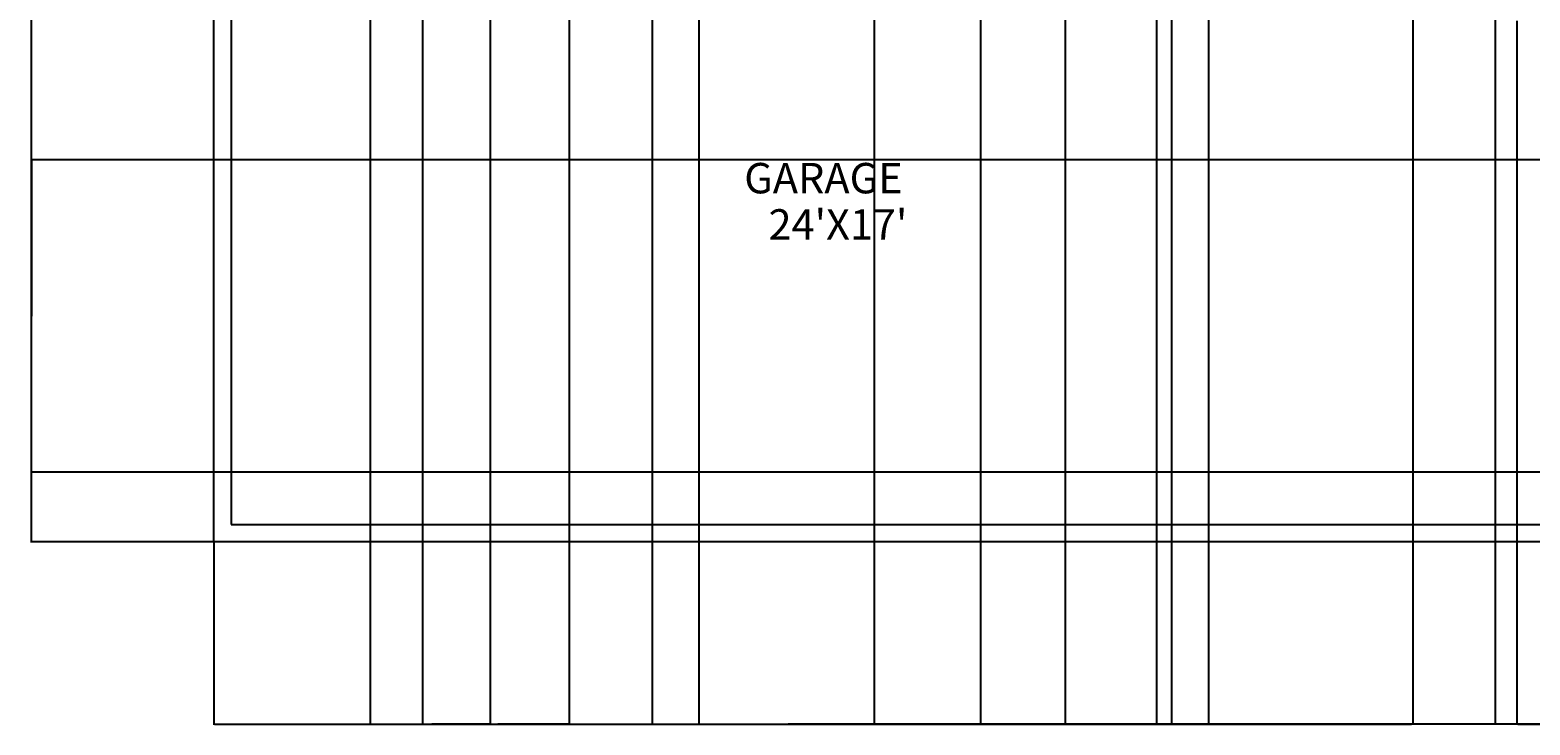
# Model space of a CAD drawing. Units: inches. Extents: x 2863 to 3499, y 1212 to 2136.
# Tile 1 of 7: x 2863 to 3208, y 1212 to 1372. Entities that reach past the tile are written whole.
import ezdxf

# ---------------------------------------------------------------- set-up
doc = ezdxf.new("R2010")
doc.units = ezdxf.units.IN
for name, color, linetype, lineweight in [('A-ANNO-DIMS', 2, 'Continuous', 18), ('A-AREA-IDEN', 7, 'Continuous', 18), ('C-PROP', 51, 'Continuous', 25)]:
    doc.layers.add(name, color=color, linetype=linetype, lineweight=lineweight)
doc.styles.get("Standard").update_dxf_attribs({"font": 'arial.ttf'})
doc.dimstyles.get("Standard").update_dxf_attribs({"dimtxt": 0.18, "dimasz": 0.18, "dimexe": 0.18, "dimexo": 0.0625, "dimgap": 0.09, "dimtad": 0, "dimtih": 1, "dimtoh": 1, "dimdec": 4, "dimzin": 0, "dimdsep": 46, "dimtxsty": 'Standard', "dimcen": 0.09, "dimadec": 0, "dimazin": 0, "dimtfac": 1, "dimtdec": 4, "dimtofl": 0, "dimtmove": 0, "dimatfit": 3, "dimfxl": 1, "dimtolj": 1, "dimtzin": 0, "dimarcsym": 0})

# ---------------------------------------------------------------- blocks, each defined once
blk = doc.blocks.new('*D49')
at = {"layer": 'A-ANNO-DIMS', "color": 0, "lineweight": -2, "transparency": 16777216}
for p, q in [((2904.92, 1254.1), (2904.92, 1211.97)), ((3456.92, 1254.1), (3456.92, 1211.97)), ((2905.1, 1212.15), (3180.63, 1212.15)), ((3456.74, 1212.15), (3181.2, 1212.15))]:
    blk.add_line(p, q, dxfattribs=at)
at = {"layer": 'A-ANNO-DIMS', "color": 0, "transparency": 16777216}
for points in [[(2905.1, 1212.18), (2905.1, 1212.12), (2904.92, 1212.15)], [(3456.74, 1212.18), (3456.74, 1212.12), (3456.92, 1212.15)]]:
    blk.add_solid(points, dxfattribs=at)
at = {"layer": 'Defpoints', "color": 0, "transparency": 16777216}
for p in [(2904.92, 1254.17), (3456.92, 1254.17), (3456.92, 1212.15)]:
    blk.add_point(p, dxfattribs=at)
at = {"layer": 'A-ANNO-DIMS', "color": 0, "transparency": 16777216, "insert": (3180.92, 1212.15), "char_height": 0.18, "attachment_point": 5}
blk.add_mtext('\\A1;552', dxfattribs=at)
blk = doc.blocks.new('*D50')
at = {"layer": 'A-ANNO-DIMS', "color": 0, "lineweight": -2, "transparency": 16777216}
for p, q in [((2904.85, 2094.17), (2862.72, 2094.17)), ((2862.9, 2093.99), (2862.9, 1674.35)), ((2862.9, 1254.35), (2862.9, 1673.98)), ((2904.85, 1254.17), (2862.72, 1254.17))]:
    blk.add_line(p, q, dxfattribs=at)
at = {"layer": 'A-ANNO-DIMS', "color": 0, "transparency": 16777216}
for points in [[(2862.87, 2093.99), (2862.93, 2093.99), (2862.9, 2094.17)], [(2862.87, 1254.35), (2862.93, 1254.35), (2862.9, 1254.17)]]:
    blk.add_solid(points, dxfattribs=at)
at = {"layer": 'Defpoints', "color": 0, "transparency": 16777216}
for p in [(2862.9, 2094.17), (2904.92, 2094.17), (2904.92, 1254.17)]:
    blk.add_point(p, dxfattribs=at)
at = {"layer": 'A-ANNO-DIMS', "color": 0, "transparency": 16777216, "insert": (2862.9, 1674.17), "char_height": 0.18, "attachment_point": 5}
blk.add_mtext('\\A1;840', dxfattribs=at)
blk = doc.blocks.new('*D70')
at = {"layer": 'A-ANNO-DIMS', "color": 0, "lineweight": -2, "transparency": 16777216}
for p, q in [((2940.92, 1453.1), (2940.92, 1211.97)), ((3204.92, 1374.1), (3204.92, 1211.97)), ((2941.1, 1212.15), (3072.63, 1212.15)), ((3204.74, 1212.15), (3073.21, 1212.15))]:
    blk.add_line(p, q, dxfattribs=at)
at = {"layer": 'A-ANNO-DIMS', "color": 0, "transparency": 16777216}
for points in [[(2941.1, 1212.18), (2941.1, 1212.12), (2940.92, 1212.15)], [(3204.74, 1212.18), (3204.74, 1212.12), (3204.92, 1212.15)]]:
    blk.add_solid(points, dxfattribs=at)
at = {"layer": 'Defpoints', "color": 0, "transparency": 16777216}
for p in [(2940.92, 1453.17), (3204.92, 1374.17), (3204.92, 1212.15)]:
    blk.add_point(p, dxfattribs=at)
at = {"layer": 'A-ANNO-DIMS', "color": 0, "transparency": 16777216, "insert": (3072.92, 1212.15), "char_height": 0.18, "attachment_point": 5}
blk.add_mtext('\\A1;264', dxfattribs=at)
blk = doc.blocks.new('*D71')
at = {"layer": 'A-ANNO-DIMS', "color": 0, "lineweight": -2, "transparency": 16777216}
for p, q in [((3204.92, 1374.1), (3204.92, 1211.97)), ((3420.92, 1374.1), (3420.92, 1211.97)), ((3205.1, 1212.15), (3312.63, 1212.15)), ((3420.74, 1212.15), (3313.21, 1212.15))]:
    blk.add_line(p, q, dxfattribs=at)
at = {"layer": 'A-ANNO-DIMS', "color": 0, "transparency": 16777216}
for points in [[(3205.1, 1212.18), (3205.1, 1212.12), (3204.92, 1212.15)], [(3420.74, 1212.18), (3420.74, 1212.12), (3420.92, 1212.15)]]:
    blk.add_solid(points, dxfattribs=at)
at = {"layer": 'Defpoints', "color": 0, "transparency": 16777216}
for p in [(3204.92, 1374.17), (3420.92, 1374.17), (3420.92, 1212.15)]:
    blk.add_point(p, dxfattribs=at)
at = {"layer": 'A-ANNO-DIMS', "color": 0, "transparency": 16777216, "insert": (3312.92, 1212.15), "char_height": 0.18, "attachment_point": 5}
blk.add_mtext('\\A1;216', dxfattribs=at)
blk = doc.blocks.new('*D76')
at = {"layer": 'A-ANNO-DIMS', "color": 0, "lineweight": -2, "transparency": 16777216}
for p, q in [((2952.92, 1675.1), (2952.92, 1211.97)), ((3121.92, 1675.1), (3121.92, 1211.97)), ((2953.1, 1212.15), (3037.14, 1212.15)), ((3121.74, 1212.15), (3037.7, 1212.15))]:
    blk.add_line(p, q, dxfattribs=at)
at = {"layer": 'A-ANNO-DIMS', "color": 0, "transparency": 16777216}
for points in [[(2953.1, 1212.18), (2953.1, 1212.12), (2952.92, 1212.15)], [(3121.74, 1212.18), (3121.74, 1212.12), (3121.92, 1212.15)]]:
    blk.add_solid(points, dxfattribs=at)
at = {"layer": 'Defpoints', "color": 0, "transparency": 16777216}
for p in [(2952.92, 1675.17), (3121.92, 1675.17), (3121.92, 1212.15)]:
    blk.add_point(p, dxfattribs=at)
at = {"layer": 'A-ANNO-DIMS', "color": 0, "transparency": 16777216, "insert": (3037.42, 1212.15), "char_height": 0.18, "attachment_point": 5}
blk.add_mtext('\\A1;169', dxfattribs=at)
blk = doc.blocks.new('*D79')
at = {"layer": 'A-ANNO-DIMS', "color": 0, "lineweight": -2, "transparency": 16777216}
for p, q in [((3005.82, 1597.44), (3005.82, 1211.97)), ((3081.41, 1597.44), (3081.41, 1211.97)), ((3006, 1212.15), (3043.23, 1212.15)), ((3081.23, 1212.15), (3044.01, 1212.15))]:
    blk.add_line(p, q, dxfattribs=at)
at = {"layer": 'A-ANNO-DIMS', "color": 0, "transparency": 16777216}
for points in [[(3006, 1212.18), (3006, 1212.12), (3005.82, 1212.15)], [(3081.23, 1212.18), (3081.23, 1212.12), (3081.41, 1212.15)]]:
    blk.add_solid(points, dxfattribs=at)
at = {"layer": 'Defpoints', "color": 0, "transparency": 16777216}
for p in [(3005.82, 1597.5), (3081.41, 1597.5), (3081.41, 1212.15)]:
    blk.add_point(p, dxfattribs=at)
at = {"layer": 'A-ANNO-DIMS', "color": 0, "transparency": 16777216, "insert": (3043.62, 1212.15), "char_height": 0.18, "attachment_point": 5}
blk.add_mtext('\\A1;75.59', dxfattribs=at)
blk = doc.blocks.new('*D81')
at = {"layer": 'A-ANNO-DIMS', "color": 0, "lineweight": -2, "transparency": 16777216}
for p, q in [((3133.92, 1453.1), (3133.92, 1211.97)), ((3199.92, 1453.1), (3199.92, 1211.97)), ((3134.1, 1212.15), (3166.7, 1212.15)), ((3199.74, 1212.15), (3167.14, 1212.15))]:
    blk.add_line(p, q, dxfattribs=at)
at = {"layer": 'A-ANNO-DIMS', "color": 0, "transparency": 16777216}
for points in [[(3134.1, 1212.18), (3134.1, 1212.12), (3133.92, 1212.15)], [(3199.74, 1212.18), (3199.74, 1212.12), (3199.92, 1212.15)]]:
    blk.add_solid(points, dxfattribs=at)
at = {"layer": 'Defpoints', "color": 0, "transparency": 16777216}
for p in [(3133.92, 1453.17), (3199.92, 1453.17), (3199.92, 1212.15)]:
    blk.add_point(p, dxfattribs=at)
at = {"layer": 'A-ANNO-DIMS', "color": 0, "transparency": 16777216, "insert": (3166.92, 1212.15), "char_height": 0.18, "attachment_point": 5}
blk.add_mtext('\\A1;66', dxfattribs=at)
blk = doc.blocks.new('*D101')
at = {"layer": 'A-ANNO-DIMS', "color": 0, "lineweight": -2, "transparency": 16777216}
for p, q in [((2940.92, 1453.1), (2940.92, 1211.97)), ((2968.53, 1453.1), (2968.53, 1211.97)), ((2941.1, 1212.15), (2954.34, 1212.15)), ((2968.35, 1212.15), (2955.1, 1212.15))]:
    blk.add_line(p, q, dxfattribs=at)
at = {"layer": 'A-ANNO-DIMS', "color": 0, "transparency": 16777216}
for points in [[(2941.1, 1212.18), (2941.1, 1212.12), (2940.92, 1212.15)], [(2968.35, 1212.18), (2968.35, 1212.12), (2968.53, 1212.15)]]:
    blk.add_solid(points, dxfattribs=at)
at = {"layer": 'Defpoints', "color": 0, "transparency": 16777216}
for p in [(2940.92, 1453.17), (2968.53, 1453.17), (2968.53, 1212.15)]:
    blk.add_point(p, dxfattribs=at)
at = {"layer": 'A-ANNO-DIMS', "color": 0, "transparency": 16777216, "insert": (2954.72, 1212.15), "char_height": 0.18, "attachment_point": 5}
blk.add_mtext('\\A1;27.61', dxfattribs=at)
blk = doc.blocks.new('*D102')
at = {"layer": 'A-ANNO-DIMS', "color": 0, "lineweight": -2, "transparency": 16777216}
for p, q in [((3016.53, 1453.1), (3016.53, 1211.97)), ((3056.9, 1453.1), (3056.9, 1211.97)), ((3016.71, 1212.15), (3036.31, 1212.15)), ((3056.72, 1212.15), (3037.11, 1212.15))]:
    blk.add_line(p, q, dxfattribs=at)
at = {"layer": 'A-ANNO-DIMS', "color": 0, "transparency": 16777216}
for points in [[(3016.71, 1212.18), (3016.71, 1212.12), (3016.53, 1212.15)], [(3056.72, 1212.18), (3056.72, 1212.12), (3056.9, 1212.15)]]:
    blk.add_solid(points, dxfattribs=at)
at = {"layer": 'Defpoints', "color": 0, "transparency": 16777216}
for p in [(3016.53, 1453.17), (3056.9, 1453.17), (3056.9, 1212.15)]:
    blk.add_point(p, dxfattribs=at)
at = {"layer": 'A-ANNO-DIMS', "color": 0, "transparency": 16777216, "insert": (3036.71, 1212.15), "char_height": 0.18, "attachment_point": 5}
blk.add_mtext('\\A1;40.37', dxfattribs=at)
blk = doc.blocks.new('*D103')
at = {"layer": 'A-ANNO-DIMS', "color": 0, "lineweight": -2, "transparency": 16777216}
for p, q in [((3100.9, 1453.1), (3100.9, 1211.97)), ((3133.92, 1453.1), (3133.92, 1211.97)), ((3101.08, 1212.15), (3117.01, 1212.15)), ((3133.74, 1212.15), (3117.8, 1212.15))]:
    blk.add_line(p, q, dxfattribs=at)
at = {"layer": 'A-ANNO-DIMS', "color": 0, "transparency": 16777216}
for points in [[(3101.08, 1212.18), (3101.08, 1212.12), (3100.9, 1212.15)], [(3133.74, 1212.18), (3133.74, 1212.12), (3133.92, 1212.15)]]:
    blk.add_solid(points, dxfattribs=at)
at = {"layer": 'Defpoints', "color": 0, "transparency": 16777216}
for p in [(3100.9, 1453.17), (3133.92, 1453.17), (3133.92, 1212.15)]:
    blk.add_point(p, dxfattribs=at)
at = {"layer": 'A-ANNO-DIMS', "color": 0, "transparency": 16777216, "insert": (3117.41, 1212.15), "char_height": 0.18, "attachment_point": 5}
blk.add_mtext('\\A1;33.02', dxfattribs=at)
blk = doc.blocks.new('*D108')
at = {"layer": 'A-ANNO-DIMS', "color": 0, "lineweight": -2, "transparency": 16777216}
for p, q in [((3440.85, 1342.09), (2862.72, 1342.09)), ((2862.9, 1341.91), (2862.9, 1306.31)), ((2862.9, 1270.35), (2862.9, 1305.95)), ((3440.85, 1270.17), (2862.72, 1270.17))]:
    blk.add_line(p, q, dxfattribs=at)
at = {"layer": 'A-ANNO-DIMS', "color": 0, "transparency": 16777216}
for points in [[(2862.87, 1341.91), (2862.93, 1341.91), (2862.9, 1342.09)], [(2862.87, 1270.35), (2862.93, 1270.35), (2862.9, 1270.17)]]:
    blk.add_solid(points, dxfattribs=at)
at = {"layer": 'Defpoints', "color": 0, "transparency": 16777216}
for p in [(2862.9, 1342.09), (3440.92, 1342.09), (3440.92, 1270.17)]:
    blk.add_point(p, dxfattribs=at)
at = {"layer": 'A-ANNO-DIMS', "color": 0, "transparency": 16777216, "insert": (2862.9, 1306.13), "char_height": 0.18, "attachment_point": 5}
blk.add_mtext('\\A1;71.93', dxfattribs=at)
blk = doc.blocks.new('*D109')
at = {"layer": 'A-ANNO-DIMS', "color": 0, "lineweight": -2, "transparency": 16777216}
for p, q in [((3125.36, 1429.1), (3125.36, 1211.97)), ((3180.92, 1429.1), (3180.92, 1211.97)), ((3125.54, 1212.15), (3152.74, 1212.15)), ((3180.74, 1212.15), (3153.53, 1212.15))]:
    blk.add_line(p, q, dxfattribs=at)
at = {"layer": 'A-ANNO-DIMS', "color": 0, "transparency": 16777216}
for points in [[(3125.54, 1212.18), (3125.54, 1212.12), (3125.36, 1212.15)], [(3180.74, 1212.18), (3180.74, 1212.12), (3180.92, 1212.15)]]:
    blk.add_solid(points, dxfattribs=at)
at = {"layer": 'Defpoints', "color": 0, "transparency": 16777216}
for p in [(3125.36, 1429.17), (3180.92, 1429.17), (3180.92, 1212.15)]:
    blk.add_point(p, dxfattribs=at)
at = {"layer": 'A-ANNO-DIMS', "color": 0, "transparency": 16777216, "insert": (3153.14, 1212.15), "char_height": 0.18, "attachment_point": 5}
blk.add_mtext('\\A1;55.56', dxfattribs=at)
blk = doc.blocks.new('*D112')
at = {"layer": 'A-ANNO-DIMS', "color": 0, "lineweight": -2, "transparency": 16777216}
for p, q in [((2952.92, 1800.1), (2952.92, 1211.97)), ((2986.74, 1800.1), (2986.74, 1211.97)), ((2953.1, 1212.15), (2969.37, 1212.15)), ((2986.56, 1212.15), (2970.29, 1212.15))]:
    blk.add_line(p, q, dxfattribs=at)
at = {"layer": 'A-ANNO-DIMS', "color": 0, "transparency": 16777216}
for points in [[(2953.1, 1212.18), (2953.1, 1212.12), (2952.92, 1212.15)], [(2986.56, 1212.18), (2986.56, 1212.12), (2986.74, 1212.15)]]:
    blk.add_solid(points, dxfattribs=at)
at = {"layer": 'Defpoints', "color": 0, "transparency": 16777216}
for p in [(2952.92, 1800.17), (2986.74, 1800.17), (2986.74, 1212.15)]:
    blk.add_point(p, dxfattribs=at)
at = {"layer": 'A-ANNO-DIMS', "color": 0, "transparency": 16777216, "insert": (2969.83, 1212.15), "char_height": 0.18, "attachment_point": 5}
blk.add_mtext('\\A1;33.825', dxfattribs=at)

msp = doc.modelspace()

# ---------------------------------------------------------------- linework, layer by layer
at = {"layer": 'C-PROP'}
for p, q in [((2904.9168, 1254.1651), (2904.9168, 2094.1651)), ((2908.9168, 2094.1651), (2908.9168, 1258.1651)), ((2908.9168, 1258.1651), (3452.9168, 1258.1651)), ((3456.9168, 1254.1651), (2904.9168, 1254.1651))]:
    msp.add_line(p, q, dxfattribs=at)

# ---------------------------------------------------------------- texts
at = {"layer": 'A-AREA-IDEN'}
for tag, p in [('GARAGE', (3027.0174, 1334.4024)), ("24'X17'", (3032.6113, 1323.7486))]:
    msp.add_attdef(tag, p, '', height=7, dxfattribs=at)

# ---------------------------------------------------------------- dimensions: what is measured, and where the dimension line sits
at = {"layer": 'A-ANNO-DIMS'}
for base, p1, p2, override, picture, middle in [((2862.8968, 2094.1651), (2904.9168, 1254.1651), (2904.9168, 2094.1651), {"dimdec": 0, "dimlfac": 1, "dimrnd": 0, "dimzin": 0, "dimdsep": 46, "dimlunit": 2}, '*D50', (2862.8968, 1674.1651)), ((2862.8968, 1342.0939), (3440.9168, 1270.1651), (3440.9168, 1342.0939), {"dimdec": 2, "dimlfac": 1, "dimrnd": 0, "dimzin": 0, "dimdsep": 46, "dimlunit": 2}, '*D108', (2862.8968, 1306.1295))]:
    dim = msp.add_linear_dim(base=base, p1=p1, p2=p2, angle=90, dimstyle='Standard', override=override, dxfattribs=at)
    dim.commit()
    dim.dimension.update_dxf_attribs({"geometry": picture, "text_midpoint": middle})
for base, p1, p2, override, picture, middle in [((2986.7418, 1212.1451), (2952.9168, 1800.1651), (2986.7418, 1800.1651), {"dimdec": 3, "dimlfac": 1, "dimrnd": 0, "dimzin": 0, "dimdsep": 46, "dimlunit": 2}, '*D112', (2969.8293, 1212.1451)), ((3121.9168, 1212.1451), (2952.9168, 1675.1651), (3121.9168, 1675.1651), {"dimdec": 0, "dimlfac": 1, "dimrnd": 0, "dimzin": 0, "dimdsep": 46, "dimlunit": 2}, '*D76', (3037.4168, 1212.1451)), ((3081.415, 1212.1451), (3005.8227, 1597.4979), (3081.415, 1597.4979), {"dimdec": 2, "dimlfac": 1, "dimrnd": 0, "dimzin": 0, "dimdsep": 46, "dimlunit": 2}, '*D79', (3043.6188, 1212.1451)), ((3204.9168, 1212.1451), (2940.9168, 1453.1651), (3204.9168, 1374.1651), {"dimdec": 0, "dimlfac": 1, "dimrnd": 0, "dimzin": 0, "dimdsep": 46, "dimlunit": 2}, '*D70', (3072.9168, 1212.1451)), ((2968.5255, 1212.1451), (2940.9168, 1453.1651), (2968.5255, 1453.1651), {"dimdec": 2, "dimlfac": 1, "dimrnd": 0, "dimzin": 0, "dimdsep": 46, "dimlunit": 2}, '*D101', (2954.7211, 1212.1451)), ((3056.8973, 1212.1451), (3016.5255, 1453.1651), (3056.8973, 1453.1651), {"dimdec": 2, "dimlfac": 1, "dimrnd": 0, "dimzin": 0, "dimdsep": 46, "dimlunit": 2}, '*D102', (3036.7114, 1212.1451)), ((3133.9168, 1212.1451), (3100.8973, 1453.1651), (3133.9168, 1453.1651), {"dimdec": 2, "dimlfac": 1, "dimrnd": 0, "dimzin": 0, "dimdsep": 46, "dimlunit": 2}, '*D103', (3117.407, 1212.1451)), ((3199.9168, 1212.1451), (3133.9168, 1453.1651), (3199.9168, 1453.1651), {"dimdec": 0, "dimlfac": 1, "dimrnd": 0, "dimzin": 0, "dimdsep": 46, "dimlunit": 2}, '*D81', (3166.9168, 1212.1451)), ((3180.9168, 1212.1451), (3125.3565, 1429.1651), (3180.9168, 1429.1651), {"dimdec": 2, "dimlfac": 1, "dimrnd": 0, "dimzin": 0, "dimdsep": 46, "dimlunit": 2}, '*D109', (3153.1366, 1212.1451)), ((3420.9168, 1212.1451), (3204.9168, 1374.1651), (3420.9168, 1374.1651), {"dimdec": 0, "dimlfac": 1, "dimrnd": 0, "dimzin": 0, "dimdsep": 46, "dimlunit": 2}, '*D71', (3312.9168, 1212.1451)), ((3456.9168, 1212.1451), (2904.9168, 1254.1651), (3456.9168, 1254.1651), {"dimdec": 0, "dimlfac": 1, "dimrnd": 0, "dimzin": 0, "dimdsep": 46, "dimlunit": 2}, '*D49', (3180.9168, 1212.1451))]:
    dim = msp.add_linear_dim(base=base, p1=p1, p2=p2, dimstyle='Standard', override=override, dxfattribs=at)
    dim.commit()
    dim.dimension.update_dxf_attribs({"geometry": picture, "text_midpoint": middle})

doc.saveas('drawing.dxf')
